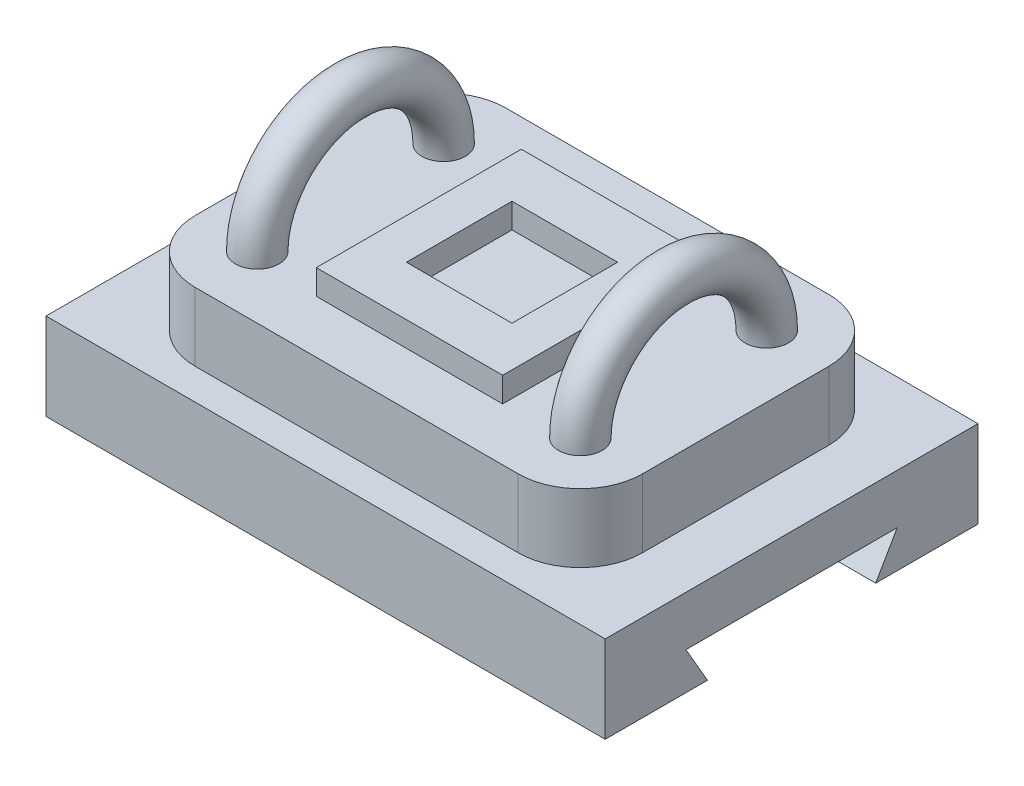
ISO-10303-21;
HEADER;
FILE_DESCRIPTION(('STEP AP214'),'2;1');
FILE_NAME('part.step','',(''),(''),'','','');
FILE_SCHEMA(('AUTOMOTIVE_DESIGN { 1 0 10303 214 1 1 1 1 }'));
ENDSEC;
DATA;
#1=APPLICATION_CONTEXT('core data for automotive mechanical design processes');
#2=APPLICATION_PROTOCOL_DEFINITION('international standard','automotive_design',2000,#1);
#3=PRODUCT_CONTEXT('',#1,'mechanical');
#4=PRODUCT('Part','Part','',(#3));
#5=PRODUCT_RELATED_PRODUCT_CATEGORY('part','',(#4));
#6=PRODUCT_DEFINITION_FORMATION('','',#4);
#7=PRODUCT_DEFINITION_CONTEXT('part definition',#1,'design');
#8=PRODUCT_DEFINITION('design','',#6,#7);
#9=PRODUCT_DEFINITION_SHAPE('','',#8);
#10=(LENGTH_UNIT() NAMED_UNIT(*) SI_UNIT(.MILLI.,.METRE.));
#11=(NAMED_UNIT(*) PLANE_ANGLE_UNIT() SI_UNIT($,.RADIAN.));
#12=(NAMED_UNIT(*) SI_UNIT($,.STERADIAN.) SOLID_ANGLE_UNIT());
#13=UNCERTAINTY_MEASURE_WITH_UNIT(LENGTH_MEASURE(1.E-05),#10,'distance_accuracy_value','');
#14=(GEOMETRIC_REPRESENTATION_CONTEXT(3) GLOBAL_UNCERTAINTY_ASSIGNED_CONTEXT((#13)) GLOBAL_UNIT_ASSIGNED_CONTEXT((#10,
#11,#12)) REPRESENTATION_CONTEXT('',''));
#15=CARTESIAN_POINT('',(0.,0.,0.));
#16=DIRECTION('',(0.,0.,1.));
#17=DIRECTION('',(1.,0.,0.));
#18=AXIS2_PLACEMENT_3D('',#15,#16,#17);
#19=CARTESIAN_POINT('',(-130.,125.,75.));
#20=DIRECTION('',(0.,-1.,0.));
#21=DIRECTION('',(0.,0.,-1.));
#22=AXIS2_PLACEMENT_3D('',#19,#20,#21);
#23=PLANE('',#22);
#24=CARTESIAN_POINT('',(-130.,125.,75.));
#25=DIRECTION('',(0.,-1.,0.));
#26=DIRECTION('',(0.,0.,1.));
#27=AXIS2_PLACEMENT_3D('',#24,#25,#26);
#28=CIRCLE('',#27,17.5);
#29=CARTESIAN_POINT('',(-130.,125.,92.5));
#30=VERTEX_POINT('',#29);
#31=EDGE_CURVE('E580',#30,#30,#28,.F.);
#32=ORIENTED_EDGE('',*,*,#31,.F.);
#33=EDGE_LOOP('',(#32));
#34=FACE_BOUND('',#33,.T.);
#35=CARTESIAN_POINT('',(-130.,125.,-75.));
#36=DIRECTION('',(0.,1.,0.));
#37=DIRECTION('',(0.,0.,-1.));
#38=AXIS2_PLACEMENT_3D('',#35,#36,#37);
#39=CIRCLE('',#38,17.5);
#40=CARTESIAN_POINT('',(-130.,125.,-92.5));
#41=VERTEX_POINT('',#40);
#42=EDGE_CURVE('E577',#41,#41,#39,.F.);
#43=ORIENTED_EDGE('',*,*,#42,.T.);
#44=EDGE_LOOP('',(#43));
#45=FACE_BOUND('',#44,.T.);
#46=CARTESIAN_POINT('',(130.,125.,75.));
#47=DIRECTION('',(0.,1.,0.));
#48=DIRECTION('',(0.,0.,1.));
#49=AXIS2_PLACEMENT_3D('',#46,#47,#48);
#50=CIRCLE('',#49,17.5);
#51=CARTESIAN_POINT('',(130.,125.,92.5));
#52=VERTEX_POINT('',#51);
#53=EDGE_CURVE('E578',#52,#52,#50,.T.);
#54=ORIENTED_EDGE('',*,*,#53,.F.);
#55=EDGE_LOOP('',(#54));
#56=FACE_BOUND('',#55,.T.);
#57=CARTESIAN_POINT('',(130.,125.,-75.));
#58=DIRECTION('',(0.,-1.,0.));
#59=DIRECTION('',(0.,0.,-1.));
#60=AXIS2_PLACEMENT_3D('',#57,#58,#59);
#61=CIRCLE('',#60,17.5);
#62=CARTESIAN_POINT('',(130.,125.,-92.5));
#63=VERTEX_POINT('',#62);
#64=EDGE_CURVE('E245',#63,#63,#61,.T.);
#65=ORIENTED_EDGE('',*,*,#64,.T.);
#66=EDGE_LOOP('',(#65));
#67=FACE_BOUND('',#66,.T.);
#68=CARTESIAN_POINT('',(-130.,125.,75.));
#69=DIRECTION('',(0.,1.,0.));
#70=DIRECTION('',(0.,0.,-1.));
#71=AXIS2_PLACEMENT_3D('',#68,#69,#70);
#72=CIRCLE('',#71,50.);
#73=CARTESIAN_POINT('',(-180.,125.,75.));
#74=VERTEX_POINT('',#73);
#75=CARTESIAN_POINT('',(-130.,125.,125.));
#76=VERTEX_POINT('',#75);
#77=EDGE_CURVE('E287',#74,#76,#72,.T.);
#78=ORIENTED_EDGE('',*,*,#77,.T.);
#79=DIRECTION('',(1.,0.,0.));
#80=VECTOR('',#79,1.);
#81=CARTESIAN_POINT('',(-130.,125.,125.));
#82=LINE('',#81,#80);
#83=CARTESIAN_POINT('',(130.,125.,125.));
#84=VERTEX_POINT('',#83);
#85=EDGE_CURVE('E286',#76,#84,#82,.T.);
#86=ORIENTED_EDGE('',*,*,#85,.T.);
#87=CARTESIAN_POINT('',(130.,125.,75.));
#88=DIRECTION('',(0.,1.,0.));
#89=DIRECTION('',(0.,0.,1.));
#90=AXIS2_PLACEMENT_3D('',#87,#88,#89);
#91=CIRCLE('',#90,50.);
#92=CARTESIAN_POINT('',(180.,125.,75.));
#93=VERTEX_POINT('',#92);
#94=EDGE_CURVE('E295',#84,#93,#91,.T.);
#95=ORIENTED_EDGE('',*,*,#94,.T.);
#96=DIRECTION('',(0.,0.,-1.));
#97=VECTOR('',#96,1.);
#98=CARTESIAN_POINT('',(180.,125.,75.));
#99=LINE('',#98,#97);
#100=CARTESIAN_POINT('',(180.,125.,-75.));
#101=VERTEX_POINT('',#100);
#102=EDGE_CURVE('E294',#93,#101,#99,.T.);
#103=ORIENTED_EDGE('',*,*,#102,.T.);
#104=CARTESIAN_POINT('',(130.,125.,-75.));
#105=DIRECTION('',(0.,1.,0.));
#106=DIRECTION('',(0.,0.,-1.));
#107=AXIS2_PLACEMENT_3D('',#104,#105,#106);
#108=CIRCLE('',#107,50.);
#109=CARTESIAN_POINT('',(130.,125.,-125.));
#110=VERTEX_POINT('',#109);
#111=EDGE_CURVE('E296',#101,#110,#108,.T.);
#112=ORIENTED_EDGE('',*,*,#111,.T.);
#113=DIRECTION('',(-1.,0.,0.));
#114=VECTOR('',#113,1.);
#115=CARTESIAN_POINT('',(-130.,125.,-125.));
#116=LINE('',#115,#114);
#117=CARTESIAN_POINT('',(-130.,125.,-125.));
#118=VERTEX_POINT('',#117);
#119=EDGE_CURVE('E299',#110,#118,#116,.T.);
#120=ORIENTED_EDGE('',*,*,#119,.T.);
#121=CARTESIAN_POINT('',(-130.,125.,-75.));
#122=DIRECTION('',(0.,1.,0.));
#123=DIRECTION('',(0.,0.,-1.));
#124=AXIS2_PLACEMENT_3D('',#121,#122,#123);
#125=CIRCLE('',#124,50.);
#126=CARTESIAN_POINT('',(-180.,125.,-75.));
#127=VERTEX_POINT('',#126);
#128=EDGE_CURVE('E300',#118,#127,#125,.T.);
#129=ORIENTED_EDGE('',*,*,#128,.T.);
#130=DIRECTION('',(0.,0.,1.));
#131=VECTOR('',#130,1.);
#132=CARTESIAN_POINT('',(-180.,125.,75.));
#133=LINE('',#132,#131);
#134=EDGE_CURVE('E304',#127,#74,#133,.T.);
#135=ORIENTED_EDGE('',*,*,#134,.T.);
#136=EDGE_LOOP('',(#78,#86,#95,#103,#112,#120,#129,#135));
#137=FACE_BOUND('',#136,.T.);
#138=DIRECTION('',(0.,0.,-1.));
#139=VECTOR('',#138,1.);
#140=CARTESIAN_POINT('',(75.,125.,82.5));
#141=LINE('',#140,#139);
#142=CARTESIAN_POINT('',(75.,125.,82.5));
#143=VERTEX_POINT('',#142);
#144=CARTESIAN_POINT('',(75.,125.,-82.5));
#145=VERTEX_POINT('',#144);
#146=EDGE_CURVE('E70',#143,#145,#141,.T.);
#147=ORIENTED_EDGE('',*,*,#146,.F.);
#148=DIRECTION('',(1.,0.,0.));
#149=VECTOR('',#148,1.);
#150=CARTESIAN_POINT('',(-75.,125.,82.5));
#151=LINE('',#150,#149);
#152=CARTESIAN_POINT('',(-75.,125.,82.5));
#153=VERTEX_POINT('',#152);
#154=EDGE_CURVE('E75',#153,#143,#151,.T.);
#155=ORIENTED_EDGE('',*,*,#154,.F.);
#156=DIRECTION('',(0.,0.,1.));
#157=VECTOR('',#156,1.);
#158=CARTESIAN_POINT('',(-75.,125.,82.5));
#159=LINE('',#158,#157);
#160=CARTESIAN_POINT('',(-75.,125.,-82.5));
#161=VERTEX_POINT('',#160);
#162=EDGE_CURVE('E271',#161,#153,#159,.T.);
#163=ORIENTED_EDGE('',*,*,#162,.F.);
#164=DIRECTION('',(-1.,0.,0.));
#165=VECTOR('',#164,1.);
#166=CARTESIAN_POINT('',(-75.,125.,-82.5));
#167=LINE('',#166,#165);
#168=EDGE_CURVE('E268',#145,#161,#167,.T.);
#169=ORIENTED_EDGE('',*,*,#168,.F.);
#170=EDGE_LOOP('',(#147,#155,#163,#169));
#171=FACE_BOUND('',#170,.T.);
#172=ADVANCED_FACE('F52',(#34,#45,#56,#67,#137,#171),#23,.F.);
#173=CARTESIAN_POINT('',(225.,70.,150.));
#174=DIRECTION('',(0.,-1.,0.));
#175=DIRECTION('',(0.,0.,-1.));
#176=AXIS2_PLACEMENT_3D('',#173,#174,#175);
#177=PLANE('',#176);
#178=DIRECTION('',(0.,0.,1.));
#179=VECTOR('',#178,1.);
#180=CARTESIAN_POINT('',(-225.,70.,150.));
#181=LINE('',#180,#179);
#182=CARTESIAN_POINT('',(-225.,70.,-150.));
#183=VERTEX_POINT('',#182);
#184=CARTESIAN_POINT('',(-225.,70.,150.));
#185=VERTEX_POINT('',#184);
#186=EDGE_CURVE('E355',#183,#185,#181,.T.);
#187=ORIENTED_EDGE('',*,*,#186,.T.);
#188=DIRECTION('',(-1.,0.,0.));
#189=VECTOR('',#188,1.);
#190=CARTESIAN_POINT('',(225.,70.,150.));
#191=LINE('',#190,#189);
#192=CARTESIAN_POINT('',(225.,70.,150.));
#193=VERTEX_POINT('',#192);
#194=EDGE_CURVE('E369',#193,#185,#191,.T.);
#195=ORIENTED_EDGE('',*,*,#194,.F.);
#196=DIRECTION('',(0.,0.,1.));
#197=VECTOR('',#196,1.);
#198=CARTESIAN_POINT('',(225.,70.,150.));
#199=LINE('',#198,#197);
#200=CARTESIAN_POINT('',(225.,70.,-150.));
#201=VERTEX_POINT('',#200);
#202=EDGE_CURVE('E370',#201,#193,#199,.T.);
#203=ORIENTED_EDGE('',*,*,#202,.F.);
#204=DIRECTION('',(-1.,0.,0.));
#205=VECTOR('',#204,1.);
#206=CARTESIAN_POINT('',(225.,70.,-150.));
#207=LINE('',#206,#205);
#208=EDGE_CURVE('E390',#201,#183,#207,.T.);
#209=ORIENTED_EDGE('',*,*,#208,.T.);
#210=EDGE_LOOP('',(#187,#195,#203,#209));
#211=FACE_BOUND('',#210,.T.);
#212=CARTESIAN_POINT('',(-130.,70.,75.));
#213=DIRECTION('',(0.,1.,0.));
#214=DIRECTION('',(0.,0.,-1.));
#215=AXIS2_PLACEMENT_3D('',#212,#213,#214);
#216=CIRCLE('',#215,50.);
#217=CARTESIAN_POINT('',(-180.,70.,75.));
#218=VERTEX_POINT('',#217);
#219=CARTESIAN_POINT('',(-130.,70.,125.));
#220=VERTEX_POINT('',#219);
#221=EDGE_CURVE('E285',#218,#220,#216,.T.);
#222=ORIENTED_EDGE('',*,*,#221,.F.);
#223=DIRECTION('',(0.,0.,1.));
#224=VECTOR('',#223,1.);
#225=CARTESIAN_POINT('',(-180.,70.,75.));
#226=LINE('',#225,#224);
#227=CARTESIAN_POINT('',(-180.,70.,-75.));
#228=VERTEX_POINT('',#227);
#229=EDGE_CURVE('E288',#228,#218,#226,.T.);
#230=ORIENTED_EDGE('',*,*,#229,.F.);
#231=CARTESIAN_POINT('',(-130.,70.,-75.));
#232=DIRECTION('',(0.,1.,0.));
#233=DIRECTION('',(0.,0.,-1.));
#234=AXIS2_PLACEMENT_3D('',#231,#232,#233);
#235=CIRCLE('',#234,50.);
#236=CARTESIAN_POINT('',(-130.,70.,-125.));
#237=VERTEX_POINT('',#236);
#238=EDGE_CURVE('E325',#237,#228,#235,.T.);
#239=ORIENTED_EDGE('',*,*,#238,.F.);
#240=DIRECTION('',(-1.,0.,0.));
#241=VECTOR('',#240,1.);
#242=CARTESIAN_POINT('',(-130.,70.,-125.));
#243=LINE('',#242,#241);
#244=CARTESIAN_POINT('',(130.,70.,-125.));
#245=VERTEX_POINT('',#244);
#246=EDGE_CURVE('E317',#245,#237,#243,.T.);
#247=ORIENTED_EDGE('',*,*,#246,.F.);
#248=CARTESIAN_POINT('',(130.,70.,-75.));
#249=DIRECTION('',(0.,1.,0.));
#250=DIRECTION('',(0.,0.,-1.));
#251=AXIS2_PLACEMENT_3D('',#248,#249,#250);
#252=CIRCLE('',#251,50.);
#253=CARTESIAN_POINT('',(180.,70.,-75.));
#254=VERTEX_POINT('',#253);
#255=EDGE_CURVE('E316',#254,#245,#252,.T.);
#256=ORIENTED_EDGE('',*,*,#255,.F.);
#257=DIRECTION('',(0.,0.,-1.));
#258=VECTOR('',#257,1.);
#259=CARTESIAN_POINT('',(180.,70.,75.));
#260=LINE('',#259,#258);
#261=CARTESIAN_POINT('',(180.,70.,75.));
#262=VERTEX_POINT('',#261);
#263=EDGE_CURVE('E311',#262,#254,#260,.T.);
#264=ORIENTED_EDGE('',*,*,#263,.F.);
#265=CARTESIAN_POINT('',(130.,70.,75.));
#266=DIRECTION('',(0.,1.,0.));
#267=DIRECTION('',(0.,0.,1.));
#268=AXIS2_PLACEMENT_3D('',#265,#266,#267);
#269=CIRCLE('',#268,50.);
#270=CARTESIAN_POINT('',(130.,70.,125.));
#271=VERTEX_POINT('',#270);
#272=EDGE_CURVE('E309',#271,#262,#269,.T.);
#273=ORIENTED_EDGE('',*,*,#272,.F.);
#274=DIRECTION('',(1.,0.,0.));
#275=VECTOR('',#274,1.);
#276=CARTESIAN_POINT('',(-130.,70.,125.));
#277=LINE('',#276,#275);
#278=EDGE_CURVE('E307',#220,#271,#277,.T.);
#279=ORIENTED_EDGE('',*,*,#278,.F.);
#280=EDGE_LOOP('',(#222,#230,#239,#247,#256,#264,#273,#279));
#281=FACE_BOUND('',#280,.T.);
#282=ADVANCED_FACE('F434',(#211,#281),#177,.F.);
#283=CARTESIAN_POINT('',(225.,70.,150.));
#284=DIRECTION('',(0.,0.,-1.));
#285=DIRECTION('',(-1.,0.,0.));
#286=AXIS2_PLACEMENT_3D('',#283,#284,#285);
#287=PLANE('',#286);
#288=DIRECTION('',(0.,-1.,0.));
#289=VECTOR('',#288,1.);
#290=CARTESIAN_POINT('',(-225.,70.,150.));
#291=LINE('',#290,#289);
#292=CARTESIAN_POINT('',(-225.,0.,150.));
#293=VERTEX_POINT('',#292);
#294=EDGE_CURVE('E348',#185,#293,#291,.T.);
#295=ORIENTED_EDGE('',*,*,#294,.T.);
#296=DIRECTION('',(-1.,0.,0.));
#297=VECTOR('',#296,1.);
#298=CARTESIAN_POINT('',(225.,0.,150.));
#299=LINE('',#298,#297);
#300=CARTESIAN_POINT('',(225.,0.,150.));
#301=VERTEX_POINT('',#300);
#302=EDGE_CURVE('E12',#301,#293,#299,.T.);
#303=ORIENTED_EDGE('',*,*,#302,.F.);
#304=DIRECTION('',(0.,-1.,0.));
#305=VECTOR('',#304,1.);
#306=CARTESIAN_POINT('',(225.,70.,150.));
#307=LINE('',#306,#305);
#308=EDGE_CURVE('E351',#193,#301,#307,.T.);
#309=ORIENTED_EDGE('',*,*,#308,.F.);
#310=ORIENTED_EDGE('',*,*,#194,.T.);
#311=EDGE_LOOP('',(#295,#303,#309,#310));
#312=FACE_BOUND('',#311,.T.);
#313=ADVANCED_FACE('F54',(#312),#287,.F.);
#314=CARTESIAN_POINT('',(225.,0.,150.));
#315=DIRECTION('',(0.,1.,0.));
#316=DIRECTION('',(0.,0.,1.));
#317=AXIS2_PLACEMENT_3D('',#314,#315,#316);
#318=PLANE('',#317);
#319=DIRECTION('',(0.,0.,-1.));
#320=VECTOR('',#319,1.);
#321=CARTESIAN_POINT('',(-225.,0.,150.));
#322=LINE('',#321,#320);
#323=CARTESIAN_POINT('',(-225.,0.,67.679491924311));
#324=VERTEX_POINT('',#323);
#325=EDGE_CURVE('E375',#293,#324,#322,.T.);
#326=ORIENTED_EDGE('',*,*,#325,.T.);
#327=DIRECTION('',(-1.,0.,0.));
#328=VECTOR('',#327,1.);
#329=CARTESIAN_POINT('',(225.,0.,67.679491924311));
#330=LINE('',#329,#328);
#331=CARTESIAN_POINT('',(225.,0.,67.679491924311));
#332=VERTEX_POINT('',#331);
#333=EDGE_CURVE('E61',#332,#324,#330,.T.);
#334=ORIENTED_EDGE('',*,*,#333,.F.);
#335=DIRECTION('',(0.,0.,-1.));
#336=VECTOR('',#335,1.);
#337=CARTESIAN_POINT('',(225.,0.,150.));
#338=LINE('',#337,#336);
#339=EDGE_CURVE('E353',#301,#332,#338,.T.);
#340=ORIENTED_EDGE('',*,*,#339,.F.);
#341=ORIENTED_EDGE('',*,*,#302,.T.);
#342=EDGE_LOOP('',(#326,#334,#340,#341));
#343=FACE_BOUND('',#342,.T.);
#344=ADVANCED_FACE('F427',(#343),#318,.F.);
#345=CARTESIAN_POINT('',(225.,0.,67.679491924311));
#346=DIRECTION('',(0.,-0.500000000000004,0.866025403784436));
#347=DIRECTION('',(0.,-0.866025403784436,-0.500000000000004));
#348=AXIS2_PLACEMENT_3D('',#345,#346,#347);
#349=PLANE('',#348);
#350=DIRECTION('',(0.,0.866025403784436,0.500000000000004));
#351=VECTOR('',#350,1.);
#352=CARTESIAN_POINT('',(-225.,0.,67.679491924311));
#353=LINE('',#352,#351);
#354=CARTESIAN_POINT('',(-225.,30.,85.));
#355=VERTEX_POINT('',#354);
#356=EDGE_CURVE('E372',#324,#355,#353,.T.);
#357=ORIENTED_EDGE('',*,*,#356,.T.);
#358=DIRECTION('',(-1.,0.,0.));
#359=VECTOR('',#358,1.);
#360=CARTESIAN_POINT('',(225.,30.,85.));
#361=LINE('',#360,#359);
#362=CARTESIAN_POINT('',(225.,30.,85.));
#363=VERTEX_POINT('',#362);
#364=EDGE_CURVE('E396',#363,#355,#361,.T.);
#365=ORIENTED_EDGE('',*,*,#364,.F.);
#366=DIRECTION('',(0.,0.866025403784436,0.500000000000004));
#367=VECTOR('',#366,1.);
#368=CARTESIAN_POINT('',(225.,0.,67.679491924311));
#369=LINE('',#368,#367);
#370=EDGE_CURVE('E359',#332,#363,#369,.T.);
#371=ORIENTED_EDGE('',*,*,#370,.F.);
#372=ORIENTED_EDGE('',*,*,#333,.T.);
#373=EDGE_LOOP('',(#357,#365,#371,#372));
#374=FACE_BOUND('',#373,.T.);
#375=ADVANCED_FACE('F406',(#374),#349,.F.);
#376=CARTESIAN_POINT('',(225.,30.,85.));
#377=DIRECTION('',(0.,1.,0.));
#378=DIRECTION('',(0.,0.,1.));
#379=AXIS2_PLACEMENT_3D('',#376,#377,#378);
#380=PLANE('',#379);
#381=DIRECTION('',(0.,0.,-1.));
#382=VECTOR('',#381,1.);
#383=CARTESIAN_POINT('',(-225.,30.,85.));
#384=LINE('',#383,#382);
#385=CARTESIAN_POINT('',(-225.,30.,-85.));
#386=VERTEX_POINT('',#385);
#387=EDGE_CURVE('E376',#355,#386,#384,.T.);
#388=ORIENTED_EDGE('',*,*,#387,.T.);
#389=DIRECTION('',(-1.,0.,0.));
#390=VECTOR('',#389,1.);
#391=CARTESIAN_POINT('',(225.,30.,-85.));
#392=LINE('',#391,#390);
#393=CARTESIAN_POINT('',(225.,30.,-85.));
#394=VERTEX_POINT('',#393);
#395=EDGE_CURVE('E397',#394,#386,#392,.T.);
#396=ORIENTED_EDGE('',*,*,#395,.F.);
#397=DIRECTION('',(0.,0.,-1.));
#398=VECTOR('',#397,1.);
#399=CARTESIAN_POINT('',(225.,30.,85.));
#400=LINE('',#399,#398);
#401=EDGE_CURVE('E356',#363,#394,#400,.T.);
#402=ORIENTED_EDGE('',*,*,#401,.F.);
#403=ORIENTED_EDGE('',*,*,#364,.T.);
#404=EDGE_LOOP('',(#388,#396,#402,#403));
#405=FACE_BOUND('',#404,.T.);
#406=ADVANCED_FACE('F417',(#405),#380,.F.);
#407=CARTESIAN_POINT('',(225.,30.,-85.));
#408=DIRECTION('',(0.,-0.500000000000004,-0.866025403784436));
#409=DIRECTION('',(0.,0.866025403784436,-0.500000000000004));
#410=AXIS2_PLACEMENT_3D('',#407,#408,#409);
#411=PLANE('',#410);
#412=DIRECTION('',(0.,-0.866025403784436,0.500000000000004));
#413=VECTOR('',#412,1.);
#414=CARTESIAN_POINT('',(-225.,30.,-85.));
#415=LINE('',#414,#413);
#416=CARTESIAN_POINT('',(-225.,0.,-67.679491924311));
#417=VERTEX_POINT('',#416);
#418=EDGE_CURVE('E378',#386,#417,#415,.T.);
#419=ORIENTED_EDGE('',*,*,#418,.T.);
#420=DIRECTION('',(-1.,0.,0.));
#421=VECTOR('',#420,1.);
#422=CARTESIAN_POINT('',(225.,0.,-67.679491924311));
#423=LINE('',#422,#421);
#424=CARTESIAN_POINT('',(225.,0.,-67.679491924311));
#425=VERTEX_POINT('',#424);
#426=EDGE_CURVE('E394',#425,#417,#423,.T.);
#427=ORIENTED_EDGE('',*,*,#426,.F.);
#428=DIRECTION('',(0.,-0.866025403784436,0.500000000000004));
#429=VECTOR('',#428,1.);
#430=CARTESIAN_POINT('',(225.,30.,-85.));
#431=LINE('',#430,#429);
#432=EDGE_CURVE('E363',#394,#425,#431,.T.);
#433=ORIENTED_EDGE('',*,*,#432,.F.);
#434=ORIENTED_EDGE('',*,*,#395,.T.);
#435=EDGE_LOOP('',(#419,#427,#433,#434));
#436=FACE_BOUND('',#435,.T.);
#437=ADVANCED_FACE('F423',(#436),#411,.F.);
#438=CARTESIAN_POINT('',(225.,0.,-67.679491924311));
#439=DIRECTION('',(0.,1.,0.));
#440=DIRECTION('',(0.,0.,1.));
#441=AXIS2_PLACEMENT_3D('',#438,#439,#440);
#442=PLANE('',#441);
#443=DIRECTION('',(0.,0.,-1.));
#444=VECTOR('',#443,1.);
#445=CARTESIAN_POINT('',(-225.,0.,-67.679491924311));
#446=LINE('',#445,#444);
#447=CARTESIAN_POINT('',(-225.,0.,-150.));
#448=VERTEX_POINT('',#447);
#449=EDGE_CURVE('E379',#417,#448,#446,.T.);
#450=ORIENTED_EDGE('',*,*,#449,.T.);
#451=DIRECTION('',(-1.,0.,0.));
#452=VECTOR('',#451,1.);
#453=CARTESIAN_POINT('',(225.,0.,-150.));
#454=LINE('',#453,#452);
#455=CARTESIAN_POINT('',(225.,0.,-150.));
#456=VERTEX_POINT('',#455);
#457=EDGE_CURVE('E388',#456,#448,#454,.T.);
#458=ORIENTED_EDGE('',*,*,#457,.F.);
#459=DIRECTION('',(0.,0.,-1.));
#460=VECTOR('',#459,1.);
#461=CARTESIAN_POINT('',(225.,0.,-67.679491924311));
#462=LINE('',#461,#460);
#463=EDGE_CURVE('E361',#425,#456,#462,.T.);
#464=ORIENTED_EDGE('',*,*,#463,.F.);
#465=ORIENTED_EDGE('',*,*,#426,.T.);
#466=EDGE_LOOP('',(#450,#458,#464,#465));
#467=FACE_BOUND('',#466,.T.);
#468=ADVANCED_FACE('F444',(#467),#442,.F.);
#469=CARTESIAN_POINT('',(225.,70.,-150.));
#470=DIRECTION('',(0.,0.,1.));
#471=DIRECTION('',(1.,0.,0.));
#472=AXIS2_PLACEMENT_3D('',#469,#470,#471);
#473=PLANE('',#472);
#474=DIRECTION('',(0.,1.,0.));
#475=VECTOR('',#474,1.);
#476=CARTESIAN_POINT('',(-225.,70.,-150.));
#477=LINE('',#476,#475);
#478=EDGE_CURVE('E385',#448,#183,#477,.T.);
#479=ORIENTED_EDGE('',*,*,#478,.T.);
#480=ORIENTED_EDGE('',*,*,#208,.F.);
#481=DIRECTION('',(0.,1.,0.));
#482=VECTOR('',#481,1.);
#483=CARTESIAN_POINT('',(225.,70.,-150.));
#484=LINE('',#483,#482);
#485=EDGE_CURVE('E364',#456,#201,#484,.T.);
#486=ORIENTED_EDGE('',*,*,#485,.F.);
#487=ORIENTED_EDGE('',*,*,#457,.T.);
#488=EDGE_LOOP('',(#479,#480,#486,#487));
#489=FACE_BOUND('',#488,.T.);
#490=ADVANCED_FACE('F442',(#489),#473,.F.);
#491=CARTESIAN_POINT('',(225.,0.,0.));
#492=DIRECTION('',(1.,0.,0.));
#493=DIRECTION('',(0.,0.,-1.));
#494=AXIS2_PLACEMENT_3D('',#491,#492,#493);
#495=PLANE('',#494);
#496=ORIENTED_EDGE('',*,*,#308,.T.);
#497=ORIENTED_EDGE('',*,*,#339,.T.);
#498=ORIENTED_EDGE('',*,*,#370,.T.);
#499=ORIENTED_EDGE('',*,*,#401,.T.);
#500=ORIENTED_EDGE('',*,*,#432,.T.);
#501=ORIENTED_EDGE('',*,*,#463,.T.);
#502=ORIENTED_EDGE('',*,*,#485,.T.);
#503=ORIENTED_EDGE('',*,*,#202,.T.);
#504=EDGE_LOOP('',(#496,#497,#498,#499,#500,#501,#502,#503));
#505=FACE_BOUND('',#504,.T.);
#506=ADVANCED_FACE('F422',(#505),#495,.T.);
#507=CARTESIAN_POINT('',(-225.,0.,0.));
#508=DIRECTION('',(1.,0.,0.));
#509=DIRECTION('',(0.,0.,-1.));
#510=AXIS2_PLACEMENT_3D('',#507,#508,#509);
#511=PLANE('',#510);
#512=ORIENTED_EDGE('',*,*,#294,.F.);
#513=ORIENTED_EDGE('',*,*,#186,.F.);
#514=ORIENTED_EDGE('',*,*,#478,.F.);
#515=ORIENTED_EDGE('',*,*,#449,.F.);
#516=ORIENTED_EDGE('',*,*,#418,.F.);
#517=ORIENTED_EDGE('',*,*,#387,.F.);
#518=ORIENTED_EDGE('',*,*,#356,.F.);
#519=ORIENTED_EDGE('',*,*,#325,.F.);
#520=EDGE_LOOP('',(#512,#513,#514,#515,#516,#517,#518,#519));
#521=FACE_BOUND('',#520,.T.);
#522=ADVANCED_FACE('F414',(#521),#511,.F.);
#523=CARTESIAN_POINT('',(-130.,125.,75.));
#524=DIRECTION('',(0.,-1.,0.));
#525=DIRECTION('',(0.,0.,-1.));
#526=AXIS2_PLACEMENT_3D('',#523,#524,#525);
#527=CYLINDRICAL_SURFACE('',#526,50.);
#528=ORIENTED_EDGE('',*,*,#221,.T.);
#529=DIRECTION('',(0.,-1.,0.));
#530=VECTOR('',#529,1.);
#531=CARTESIAN_POINT('',(-130.,125.,125.));
#532=LINE('',#531,#530);
#533=EDGE_CURVE('E350',#76,#220,#532,.T.);
#534=ORIENTED_EDGE('',*,*,#533,.F.);
#535=ORIENTED_EDGE('',*,*,#77,.F.);
#536=DIRECTION('',(0.,-1.,0.));
#537=VECTOR('',#536,1.);
#538=CARTESIAN_POINT('',(-180.,125.,75.));
#539=LINE('',#538,#537);
#540=EDGE_CURVE('E301',#74,#218,#539,.T.);
#541=ORIENTED_EDGE('',*,*,#540,.T.);
#542=EDGE_LOOP('',(#528,#534,#535,#541));
#543=FACE_BOUND('',#542,.T.);
#544=ADVANCED_FACE('F600',(#543),#527,.T.);
#545=CARTESIAN_POINT('',(-130.,125.,125.));
#546=DIRECTION('',(0.,0.,-1.));
#547=DIRECTION('',(-1.,0.,0.));
#548=AXIS2_PLACEMENT_3D('',#545,#546,#547);
#549=PLANE('',#548);
#550=ORIENTED_EDGE('',*,*,#278,.T.);
#551=DIRECTION('',(0.,-1.,0.));
#552=VECTOR('',#551,1.);
#553=CARTESIAN_POINT('',(130.,125.,125.));
#554=LINE('',#553,#552);
#555=EDGE_CURVE('E341',#84,#271,#554,.T.);
#556=ORIENTED_EDGE('',*,*,#555,.F.);
#557=ORIENTED_EDGE('',*,*,#85,.F.);
#558=ORIENTED_EDGE('',*,*,#533,.T.);
#559=EDGE_LOOP('',(#550,#556,#557,#558));
#560=FACE_BOUND('',#559,.T.);
#561=ADVANCED_FACE('F597',(#560),#549,.F.);
#562=CARTESIAN_POINT('',(130.,125.,75.));
#563=DIRECTION('',(0.,-1.,0.));
#564=DIRECTION('',(0.,0.,-1.));
#565=AXIS2_PLACEMENT_3D('',#562,#563,#564);
#566=CYLINDRICAL_SURFACE('',#565,50.);
#567=ORIENTED_EDGE('',*,*,#272,.T.);
#568=DIRECTION('',(0.,-1.,0.));
#569=VECTOR('',#568,1.);
#570=CARTESIAN_POINT('',(180.,125.,75.));
#571=LINE('',#570,#569);
#572=EDGE_CURVE('E342',#93,#262,#571,.T.);
#573=ORIENTED_EDGE('',*,*,#572,.F.);
#574=ORIENTED_EDGE('',*,*,#94,.F.);
#575=ORIENTED_EDGE('',*,*,#555,.T.);
#576=EDGE_LOOP('',(#567,#573,#574,#575));
#577=FACE_BOUND('',#576,.T.);
#578=ADVANCED_FACE('F602',(#577),#566,.T.);
#579=CARTESIAN_POINT('',(180.,125.,75.));
#580=DIRECTION('',(-1.,0.,0.));
#581=DIRECTION('',(0.,0.,1.));
#582=AXIS2_PLACEMENT_3D('',#579,#580,#581);
#583=PLANE('',#582);
#584=ORIENTED_EDGE('',*,*,#263,.T.);
#585=DIRECTION('',(0.,-1.,0.));
#586=VECTOR('',#585,1.);
#587=CARTESIAN_POINT('',(180.,125.,-75.));
#588=LINE('',#587,#586);
#589=EDGE_CURVE('E339',#101,#254,#588,.T.);
#590=ORIENTED_EDGE('',*,*,#589,.F.);
#591=ORIENTED_EDGE('',*,*,#102,.F.);
#592=ORIENTED_EDGE('',*,*,#572,.T.);
#593=EDGE_LOOP('',(#584,#590,#591,#592));
#594=FACE_BOUND('',#593,.T.);
#595=ADVANCED_FACE('F606',(#594),#583,.F.);
#596=CARTESIAN_POINT('',(130.,125.,-75.));
#597=DIRECTION('',(0.,-1.,0.));
#598=DIRECTION('',(0.,0.,-1.));
#599=AXIS2_PLACEMENT_3D('',#596,#597,#598);
#600=CYLINDRICAL_SURFACE('',#599,50.);
#601=ORIENTED_EDGE('',*,*,#255,.T.);
#602=DIRECTION('',(0.,-1.,0.));
#603=VECTOR('',#602,1.);
#604=CARTESIAN_POINT('',(130.,125.,-125.));
#605=LINE('',#604,#603);
#606=EDGE_CURVE('E333',#110,#245,#605,.T.);
#607=ORIENTED_EDGE('',*,*,#606,.F.);
#608=ORIENTED_EDGE('',*,*,#111,.F.);
#609=ORIENTED_EDGE('',*,*,#589,.T.);
#610=EDGE_LOOP('',(#601,#607,#608,#609));
#611=FACE_BOUND('',#610,.T.);
#612=ADVANCED_FACE('F611',(#611),#600,.T.);
#613=CARTESIAN_POINT('',(-130.,125.,-125.));
#614=DIRECTION('',(0.,0.,1.));
#615=DIRECTION('',(1.,0.,0.));
#616=AXIS2_PLACEMENT_3D('',#613,#614,#615);
#617=PLANE('',#616);
#618=ORIENTED_EDGE('',*,*,#246,.T.);
#619=DIRECTION('',(0.,-1.,0.));
#620=VECTOR('',#619,1.);
#621=CARTESIAN_POINT('',(-130.,125.,-125.));
#622=LINE('',#621,#620);
#623=EDGE_CURVE('E335',#118,#237,#622,.T.);
#624=ORIENTED_EDGE('',*,*,#623,.F.);
#625=ORIENTED_EDGE('',*,*,#119,.F.);
#626=ORIENTED_EDGE('',*,*,#606,.T.);
#627=EDGE_LOOP('',(#618,#624,#625,#626));
#628=FACE_BOUND('',#627,.T.);
#629=ADVANCED_FACE('F615',(#628),#617,.F.);
#630=CARTESIAN_POINT('',(-130.,125.,-75.));
#631=DIRECTION('',(0.,-1.,0.));
#632=DIRECTION('',(0.,0.,-1.));
#633=AXIS2_PLACEMENT_3D('',#630,#631,#632);
#634=CYLINDRICAL_SURFACE('',#633,50.);
#635=ORIENTED_EDGE('',*,*,#238,.T.);
#636=DIRECTION('',(0.,-1.,0.));
#637=VECTOR('',#636,1.);
#638=CARTESIAN_POINT('',(-180.,125.,-75.));
#639=LINE('',#638,#637);
#640=EDGE_CURVE('E328',#127,#228,#639,.T.);
#641=ORIENTED_EDGE('',*,*,#640,.F.);
#642=ORIENTED_EDGE('',*,*,#128,.F.);
#643=ORIENTED_EDGE('',*,*,#623,.T.);
#644=EDGE_LOOP('',(#635,#641,#642,#643));
#645=FACE_BOUND('',#644,.T.);
#646=ADVANCED_FACE('F616',(#645),#634,.T.);
#647=CARTESIAN_POINT('',(-180.,125.,75.));
#648=DIRECTION('',(1.,0.,0.));
#649=DIRECTION('',(0.,0.,-1.));
#650=AXIS2_PLACEMENT_3D('',#647,#648,#649);
#651=PLANE('',#650);
#652=ORIENTED_EDGE('',*,*,#229,.T.);
#653=ORIENTED_EDGE('',*,*,#540,.F.);
#654=ORIENTED_EDGE('',*,*,#134,.F.);
#655=ORIENTED_EDGE('',*,*,#640,.T.);
#656=EDGE_LOOP('',(#652,#653,#654,#655));
#657=FACE_BOUND('',#656,.T.);
#658=ADVANCED_FACE('F493',(#657),#651,.F.);
#659=CARTESIAN_POINT('',(0.,145.,0.));
#660=DIRECTION('',(0.,-1.,0.));
#661=DIRECTION('',(0.,0.,-1.));
#662=AXIS2_PLACEMENT_3D('',#659,#660,#661);
#663=PLANE('',#662);
#664=DIRECTION('',(0.,0.,-1.));
#665=VECTOR('',#664,1.);
#666=CARTESIAN_POINT('',(75.,145.,82.5));
#667=LINE('',#666,#665);
#668=CARTESIAN_POINT('',(75.,145.,82.5));
#669=VERTEX_POINT('',#668);
#670=CARTESIAN_POINT('',(75.,145.,-82.5));
#671=VERTEX_POINT('',#670);
#672=EDGE_CURVE('E260',#669,#671,#667,.T.);
#673=ORIENTED_EDGE('',*,*,#672,.T.);
#674=DIRECTION('',(-1.,0.,0.));
#675=VECTOR('',#674,1.);
#676=CARTESIAN_POINT('',(-75.,145.,-82.5));
#677=LINE('',#676,#675);
#678=CARTESIAN_POINT('',(-75.,145.,-82.5));
#679=VERTEX_POINT('',#678);
#680=EDGE_CURVE('E257',#671,#679,#677,.T.);
#681=ORIENTED_EDGE('',*,*,#680,.T.);
#682=DIRECTION('',(0.,0.,1.));
#683=VECTOR('',#682,1.);
#684=CARTESIAN_POINT('',(-75.,145.,82.5));
#685=LINE('',#684,#683);
#686=CARTESIAN_POINT('',(-75.,145.,82.5));
#687=VERTEX_POINT('',#686);
#688=EDGE_CURVE('E265',#679,#687,#685,.T.);
#689=ORIENTED_EDGE('',*,*,#688,.T.);
#690=DIRECTION('',(1.,0.,0.));
#691=VECTOR('',#690,1.);
#692=CARTESIAN_POINT('',(-75.,145.,82.5));
#693=LINE('',#692,#691);
#694=EDGE_CURVE('E262',#687,#669,#693,.T.);
#695=ORIENTED_EDGE('',*,*,#694,.T.);
#696=EDGE_LOOP('',(#673,#681,#689,#695));
#697=FACE_BOUND('',#696,.T.);
#698=DIRECTION('',(0.,0.,-1.));
#699=VECTOR('',#698,1.);
#700=CARTESIAN_POINT('',(42.5,145.,42.5));
#701=LINE('',#700,#699);
#702=CARTESIAN_POINT('',(42.5,145.,42.5));
#703=VERTEX_POINT('',#702);
#704=CARTESIAN_POINT('',(42.5,145.,-42.5));
#705=VERTEX_POINT('',#704);
#706=EDGE_CURVE('E213',#703,#705,#701,.T.);
#707=ORIENTED_EDGE('',*,*,#706,.F.);
#708=DIRECTION('',(1.,0.,0.));
#709=VECTOR('',#708,1.);
#710=CARTESIAN_POINT('',(-42.5,145.,42.5));
#711=LINE('',#710,#709);
#712=CARTESIAN_POINT('',(-42.5,145.,42.5));
#713=VERTEX_POINT('',#712);
#714=EDGE_CURVE('E236',#713,#703,#711,.T.);
#715=ORIENTED_EDGE('',*,*,#714,.F.);
#716=DIRECTION('',(0.,0.,1.));
#717=VECTOR('',#716,1.);
#718=CARTESIAN_POINT('',(-42.5,145.,42.5));
#719=LINE('',#718,#717);
#720=CARTESIAN_POINT('',(-42.5,145.,-42.5));
#721=VERTEX_POINT('',#720);
#722=EDGE_CURVE('E237',#721,#713,#719,.T.);
#723=ORIENTED_EDGE('',*,*,#722,.F.);
#724=DIRECTION('',(-1.,0.,0.));
#725=VECTOR('',#724,1.);
#726=CARTESIAN_POINT('',(-42.5,145.,-42.5));
#727=LINE('',#726,#725);
#728=EDGE_CURVE('E224',#705,#721,#727,.T.);
#729=ORIENTED_EDGE('',*,*,#728,.F.);
#730=EDGE_LOOP('',(#707,#715,#723,#729));
#731=FACE_BOUND('',#730,.T.);
#732=ADVANCED_FACE('F231',(#697,#731),#663,.F.);
#733=CARTESIAN_POINT('',(75.,145.,82.5));
#734=DIRECTION('',(-1.,0.,0.));
#735=DIRECTION('',(0.,0.,1.));
#736=AXIS2_PLACEMENT_3D('',#733,#734,#735);
#737=PLANE('',#736);
#738=ORIENTED_EDGE('',*,*,#146,.T.);
#739=DIRECTION('',(0.,-1.,0.));
#740=VECTOR('',#739,1.);
#741=CARTESIAN_POINT('',(75.,145.,-82.5));
#742=LINE('',#741,#740);
#743=EDGE_CURVE('E282',#671,#145,#742,.T.);
#744=ORIENTED_EDGE('',*,*,#743,.F.);
#745=ORIENTED_EDGE('',*,*,#672,.F.);
#746=DIRECTION('',(0.,-1.,0.));
#747=VECTOR('',#746,1.);
#748=CARTESIAN_POINT('',(75.,145.,82.5));
#749=LINE('',#748,#747);
#750=EDGE_CURVE('E266',#669,#143,#749,.T.);
#751=ORIENTED_EDGE('',*,*,#750,.T.);
#752=EDGE_LOOP('',(#738,#744,#745,#751));
#753=FACE_BOUND('',#752,.T.);
#754=ADVANCED_FACE('F492',(#753),#737,.F.);
#755=CARTESIAN_POINT('',(-75.,145.,-82.5));
#756=DIRECTION('',(0.,0.,1.));
#757=DIRECTION('',(1.,0.,0.));
#758=AXIS2_PLACEMENT_3D('',#755,#756,#757);
#759=PLANE('',#758);
#760=ORIENTED_EDGE('',*,*,#168,.T.);
#761=DIRECTION('',(0.,-1.,0.));
#762=VECTOR('',#761,1.);
#763=CARTESIAN_POINT('',(-75.,145.,-82.5));
#764=LINE('',#763,#762);
#765=EDGE_CURVE('E276',#679,#161,#764,.T.);
#766=ORIENTED_EDGE('',*,*,#765,.F.);
#767=ORIENTED_EDGE('',*,*,#680,.F.);
#768=ORIENTED_EDGE('',*,*,#743,.T.);
#769=EDGE_LOOP('',(#760,#766,#767,#768));
#770=FACE_BOUND('',#769,.T.);
#771=ADVANCED_FACE('F502',(#770),#759,.F.);
#772=CARTESIAN_POINT('',(-75.,145.,82.5));
#773=DIRECTION('',(1.,0.,0.));
#774=DIRECTION('',(0.,0.,-1.));
#775=AXIS2_PLACEMENT_3D('',#772,#773,#774);
#776=PLANE('',#775);
#777=ORIENTED_EDGE('',*,*,#162,.T.);
#778=DIRECTION('',(0.,-1.,0.));
#779=VECTOR('',#778,1.);
#780=CARTESIAN_POINT('',(-75.,145.,82.5));
#781=LINE('',#780,#779);
#782=EDGE_CURVE('E277',#687,#153,#781,.T.);
#783=ORIENTED_EDGE('',*,*,#782,.F.);
#784=ORIENTED_EDGE('',*,*,#688,.F.);
#785=ORIENTED_EDGE('',*,*,#765,.T.);
#786=EDGE_LOOP('',(#777,#783,#784,#785));
#787=FACE_BOUND('',#786,.T.);
#788=ADVANCED_FACE('F499',(#787),#776,.F.);
#789=CARTESIAN_POINT('',(-75.,145.,82.5));
#790=DIRECTION('',(0.,0.,-1.));
#791=DIRECTION('',(-1.,0.,0.));
#792=AXIS2_PLACEMENT_3D('',#789,#790,#791);
#793=PLANE('',#792);
#794=ORIENTED_EDGE('',*,*,#154,.T.);
#795=ORIENTED_EDGE('',*,*,#750,.F.);
#796=ORIENTED_EDGE('',*,*,#694,.F.);
#797=ORIENTED_EDGE('',*,*,#782,.T.);
#798=EDGE_LOOP('',(#794,#795,#796,#797));
#799=FACE_BOUND('',#798,.T.);
#800=ADVANCED_FACE('F489',(#799),#793,.F.);
#801=CARTESIAN_POINT('',(42.5,145.,42.5));
#802=DIRECTION('',(-1.,0.,0.));
#803=DIRECTION('',(0.,0.,1.));
#804=AXIS2_PLACEMENT_3D('',#801,#802,#803);
#805=PLANE('',#804);
#806=DIRECTION('',(0.,0.,-1.));
#807=VECTOR('',#806,1.);
#808=CARTESIAN_POINT('',(42.5,125.,42.5));
#809=LINE('',#808,#807);
#810=CARTESIAN_POINT('',(42.5,125.,42.5));
#811=VERTEX_POINT('',#810);
#812=CARTESIAN_POINT('',(42.5,125.,-42.5));
#813=VERTEX_POINT('',#812);
#814=EDGE_CURVE('E244',#811,#813,#809,.T.);
#815=ORIENTED_EDGE('',*,*,#814,.F.);
#816=DIRECTION('',(0.,-1.,0.));
#817=VECTOR('',#816,1.);
#818=CARTESIAN_POINT('',(42.5,145.,42.5));
#819=LINE('',#818,#817);
#820=EDGE_CURVE('E218',#703,#811,#819,.T.);
#821=ORIENTED_EDGE('',*,*,#820,.F.);
#822=ORIENTED_EDGE('',*,*,#706,.T.);
#823=DIRECTION('',(0.,-1.,0.));
#824=VECTOR('',#823,1.);
#825=CARTESIAN_POINT('',(42.5,145.,-42.5));
#826=LINE('',#825,#824);
#827=EDGE_CURVE('E216',#705,#813,#826,.T.);
#828=ORIENTED_EDGE('',*,*,#827,.T.);
#829=EDGE_LOOP('',(#815,#821,#822,#828));
#830=FACE_BOUND('',#829,.T.);
#831=ADVANCED_FACE('F214',(#830),#805,.T.);
#832=CARTESIAN_POINT('',(-42.5,145.,-42.5));
#833=DIRECTION('',(0.,0.,1.));
#834=DIRECTION('',(1.,0.,0.));
#835=AXIS2_PLACEMENT_3D('',#832,#833,#834);
#836=PLANE('',#835);
#837=DIRECTION('',(-1.,0.,0.));
#838=VECTOR('',#837,1.);
#839=CARTESIAN_POINT('',(-42.5,125.,-42.5));
#840=LINE('',#839,#838);
#841=CARTESIAN_POINT('',(-42.5,125.,-42.5));
#842=VERTEX_POINT('',#841);
#843=EDGE_CURVE('E230',#813,#842,#840,.T.);
#844=ORIENTED_EDGE('',*,*,#843,.F.);
#845=ORIENTED_EDGE('',*,*,#827,.F.);
#846=ORIENTED_EDGE('',*,*,#728,.T.);
#847=DIRECTION('',(0.,-1.,0.));
#848=VECTOR('',#847,1.);
#849=CARTESIAN_POINT('',(-42.5,145.,-42.5));
#850=LINE('',#849,#848);
#851=EDGE_CURVE('E232',#721,#842,#850,.T.);
#852=ORIENTED_EDGE('',*,*,#851,.T.);
#853=EDGE_LOOP('',(#844,#845,#846,#852));
#854=FACE_BOUND('',#853,.T.);
#855=ADVANCED_FACE('F227',(#854),#836,.T.);
#856=CARTESIAN_POINT('',(-42.5,145.,42.5));
#857=DIRECTION('',(1.,0.,0.));
#858=DIRECTION('',(0.,0.,-1.));
#859=AXIS2_PLACEMENT_3D('',#856,#857,#858);
#860=PLANE('',#859);
#861=DIRECTION('',(0.,0.,1.));
#862=VECTOR('',#861,1.);
#863=CARTESIAN_POINT('',(-42.5,125.,42.5));
#864=LINE('',#863,#862);
#865=CARTESIAN_POINT('',(-42.5,125.,42.5));
#866=VERTEX_POINT('',#865);
#867=EDGE_CURVE('E249',#842,#866,#864,.T.);
#868=ORIENTED_EDGE('',*,*,#867,.F.);
#869=ORIENTED_EDGE('',*,*,#851,.F.);
#870=ORIENTED_EDGE('',*,*,#722,.T.);
#871=DIRECTION('',(0.,-1.,0.));
#872=VECTOR('',#871,1.);
#873=CARTESIAN_POINT('',(-42.5,145.,42.5));
#874=LINE('',#873,#872);
#875=EDGE_CURVE('E251',#713,#866,#874,.T.);
#876=ORIENTED_EDGE('',*,*,#875,.T.);
#877=EDGE_LOOP('',(#868,#869,#870,#876));
#878=FACE_BOUND('',#877,.T.);
#879=ADVANCED_FACE('F478',(#878),#860,.T.);
#880=CARTESIAN_POINT('',(-42.5,145.,42.5));
#881=DIRECTION('',(0.,0.,-1.));
#882=DIRECTION('',(-1.,0.,0.));
#883=AXIS2_PLACEMENT_3D('',#880,#881,#882);
#884=PLANE('',#883);
#885=DIRECTION('',(1.,0.,0.));
#886=VECTOR('',#885,1.);
#887=CARTESIAN_POINT('',(-42.5,125.,42.5));
#888=LINE('',#887,#886);
#889=EDGE_CURVE('E221',#866,#811,#888,.T.);
#890=ORIENTED_EDGE('',*,*,#889,.F.);
#891=ORIENTED_EDGE('',*,*,#875,.F.);
#892=ORIENTED_EDGE('',*,*,#714,.T.);
#893=ORIENTED_EDGE('',*,*,#820,.T.);
#894=EDGE_LOOP('',(#890,#891,#892,#893));
#895=FACE_BOUND('',#894,.T.);
#896=ADVANCED_FACE('F470',(#895),#884,.T.);
#897=ORIENTED_EDGE('',*,*,#867,.T.);
#898=ORIENTED_EDGE('',*,*,#889,.T.);
#899=ORIENTED_EDGE('',*,*,#814,.T.);
#900=ORIENTED_EDGE('',*,*,#843,.T.);
#901=EDGE_LOOP('',(#897,#898,#899,#900));
#902=FACE_BOUND('',#901,.T.);
#903=ADVANCED_FACE('F453',(#902),#23,.F.);
#904=CARTESIAN_POINT('',(130.,125.,0.));
#905=DIRECTION('',(-1.,0.,0.));
#906=DIRECTION('',(0.,0.,1.));
#907=AXIS2_PLACEMENT_3D('',#904,#905,#906);
#908=TOROIDAL_SURFACE('',#907,75.,17.5);
#909=CARTESIAN_POINT('',(130.,125.,0.));
#910=DIRECTION('',(-1.,0.,0.));
#911=DIRECTION('',(0.,0.,1.));
#912=AXIS2_PLACEMENT_3D('',#909,#910,#911);
#913=CIRCLE('',#912,92.5);
#914=EDGE_CURVE('',#52,#63,#913,.T.);
#915=ORIENTED_EDGE('',*,*,#53,.T.);
#916=ORIENTED_EDGE('',*,*,#64,.F.);
#917=ORIENTED_EDGE('',*,*,#914,.T.);
#918=ORIENTED_EDGE('',*,*,#914,.F.);
#919=EDGE_LOOP('',(#915,#917,#916,#918));
#920=FACE_BOUND('',#919,.T.);
#921=ADVANCED_FACE('F469',(#920),#908,.T.);
#922=CARTESIAN_POINT('',(-130.,125.,0.));
#923=DIRECTION('',(-1.,0.,0.));
#924=DIRECTION('',(0.,0.,1.));
#925=AXIS2_PLACEMENT_3D('',#922,#923,#924);
#926=TOROIDAL_SURFACE('',#925,75.,17.5);
#927=CARTESIAN_POINT('',(-130.,125.,0.));
#928=DIRECTION('',(-1.,0.,0.));
#929=DIRECTION('',(0.,0.,1.));
#930=AXIS2_PLACEMENT_3D('',#927,#928,#929);
#931=CIRCLE('',#930,92.5);
#932=EDGE_CURVE('',#30,#41,#931,.T.);
#933=ORIENTED_EDGE('',*,*,#31,.T.);
#934=ORIENTED_EDGE('',*,*,#42,.F.);
#935=ORIENTED_EDGE('',*,*,#932,.T.);
#936=ORIENTED_EDGE('',*,*,#932,.F.);
#937=EDGE_LOOP('',(#933,#935,#934,#936));
#938=FACE_BOUND('',#937,.T.);
#939=ADVANCED_FACE('F471',(#938),#926,.T.);
#940=CLOSED_SHELL('',(#172,#282,#313,#344,#375,#406,#437,#468,#490,#506,#522,#544,#561,#578,
#595,#612,#629,#646,#658,#732,#754,#771,#788,#800,#831,#855,#879,#896,#903,#921,#939));
#941=MANIFOLD_SOLID_BREP('B2',#940);
#942=ADVANCED_BREP_SHAPE_REPRESENTATION('',(#18,#941),#14);
#943=SHAPE_DEFINITION_REPRESENTATION(#9,#942);
ENDSEC;
END-ISO-10303-21;
